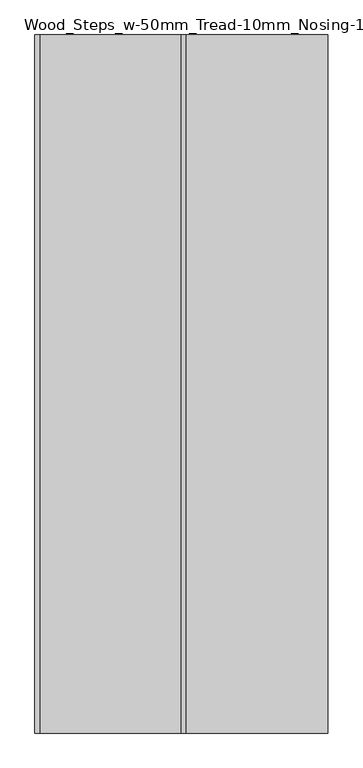
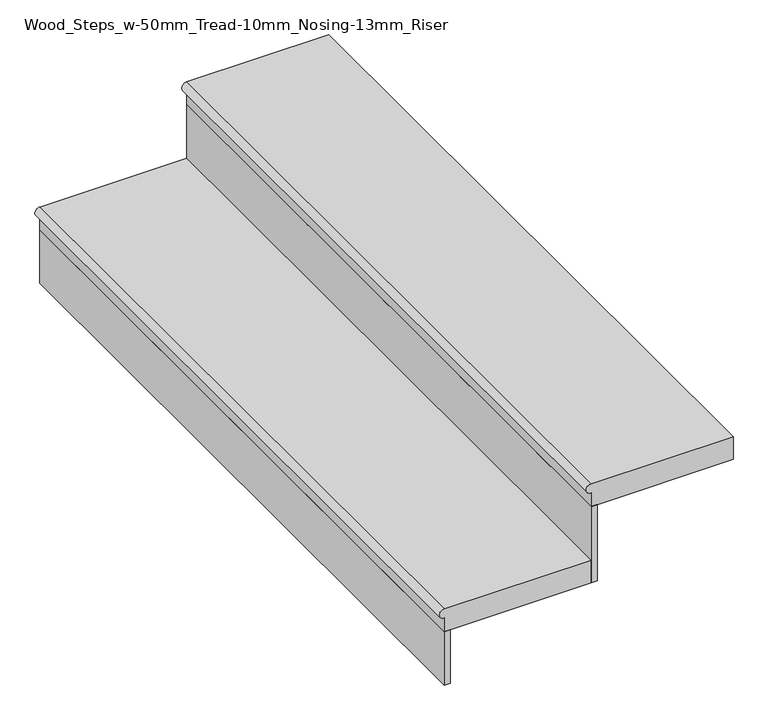
"""IFC4 building model written with IfcOpenShell, lengths in millimetres: stair flight geometry, Wood_Steps_w-50mm_Tread-10mm_Nosing-13mm_Riser."""

from ifc_helpers import new_model, si_unit, point, frame, frame_2d, origin, place, context, project, spatial, polyline, circle_curve, trimmed, segment, composite_curve, outline, extrude, source, transform, mapped, element, save


def wood_steps_w_50mm_tread_10mm_nosing_13mm_riser_13d2c295(model_context):
    return source(origin(), model_context, "Body", "SweptSolid", [
        extrude(outline(composite_curve([segment(polyline([(-137.16, -4867.8277418), (-137.16, -5172.6277418)]), True, "CONTINUOUS"), segment(trimmed(circle_curve(frame_2d((-147.16, -5172.6277418)), 10.0), [point((-137.16, -5172.6277418))], [point((-157.16, -5172.6277418))], False, "CARTESIAN"), True, "CONTINUOUS"), segment(polyline([(-157.16, -5172.6277418), (-187.16, -5172.6277418), (-187.16, -4867.8277418), (-137.16, -4867.8277418)]), True, "CONTINUOUS")], self_intersect=False)), frame((0.0, 2060.6912809, 0.0), z_axis=(0.0, 1.0, 0.0), x_axis=(0.0, 0.0, 1.0)), (0.0, 0.0, 1.0), 1453.5261162),
        extrude(outline(polyline([(-5160.1277418, 2060.6912809), (-5172.6277418, 2060.6912809), (-5172.6277418, 3514.2173971), (-5160.1277418, 3514.2173971), (-5160.1277418, 2060.6912809)])), frame((0.0, 0.0, -304.8), z_axis=(0.0, 0.0, 1.0), x_axis=(1.0, 0.0, 0.0)), (0.0, 0.0, 1.0), 117.64),
        extrude(outline(polyline([(-4855.3277418, 2060.6912809), (-4867.8277418, 2060.6912809), (-4867.8277418, 3514.2173971), (-4855.3277418, 3514.2173971), (-4855.3277418, 2060.6912809)])), frame((0.0, 0.0, -187.16), z_axis=(0.0, 0.0, 1.0), x_axis=(1.0, 0.0, 0.0)), (0.0, 0.0, 1.0), 167.64),
        extrude(outline(composite_curve([segment(polyline([(30.48, -4573.0277418), (30.48, -4867.8277418)]), True, "CONTINUOUS"), segment(trimmed(circle_curve(frame_2d((20.48, -4867.8277418)), 10.0), [point((30.48, -4867.8277418))], [point((10.48, -4867.8277418))], False, "CARTESIAN"), True, "CONTINUOUS"), segment(polyline([(10.48, -4867.8277418), (-19.52, -4867.8277418), (-19.52, -4573.0277418), (30.48, -4573.0277418)]), True, "CONTINUOUS")], self_intersect=False)), frame((0.0, 2060.6912809, 0.0), z_axis=(0.0, 1.0, 0.0), x_axis=(0.0, 0.0, 1.0)), (0.0, 0.0, 1.0), 1453.5261162),
    ])


if __name__ == "__main__":
    model = new_model("IFC4")
    model_context = context("Model", 3, world=origin())
    ifc_project = project(units=[si_unit("LENGTHUNIT", "METRE", prefix="MILLI")], contexts=[model_context])
    site = spatial("IfcSite", under=ifc_project)
    building = spatial("IfcBuilding", under=site)
    placement = place(None, origin())
    wood_steps_w_50mm_tread_10mm_nosing_13mm_riser_shape = wood_steps_w_50mm_tread_10mm_nosing_13mm_riser_13d2c295(model_context)
    element("IfcStairFlight", 1, ObjectType="Wood_Steps_w-50mm_Tread-10mm_Nosing-13mm_Riser", at=placement, inside=building, context=model_context, shape_type="MappedRepresentation", body=[
        mapped(wood_steps_w_50mm_tread_10mm_nosing_13mm_riser_shape, transform((0.0, 0.0, 0.0), x_axis=(1.0, 0.0, 0.0), y_axis=(0.0, 1.0, 0.0), z_axis=(0.0, 0.0, 1.0))),
    ])
    save(model, "model.ifc")

# Revit data of these elements
# Element 1 (IfcStairFlight, "Wood_Steps_w-50mm_Tread-10mm_Nosing-13mm_Riser")
#   Materials on its faces: "Oak Flooring"
# Materials
#   "Oak Flooring": class "Wood", colour RGB 212 179 113, transparency 0, Description = "Quercus Rubra", Cost = 0
